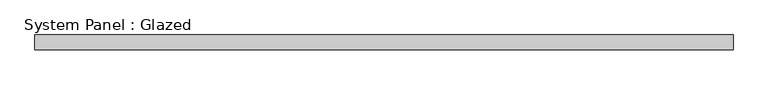
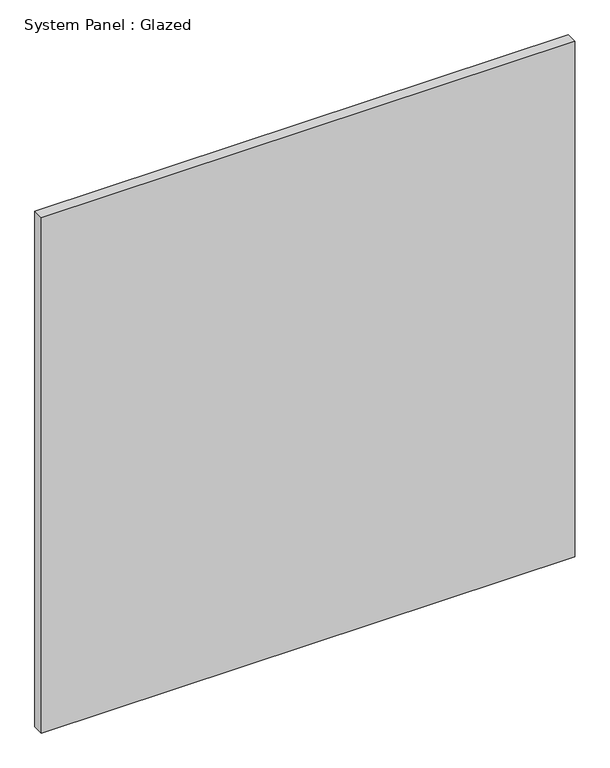
"""IFC4 building model written with IfcOpenShell, lengths in millimetres: plate geometry, System Panel : Glazed."""

from ifc_helpers import new_model, si_unit, origin, origin_with_axes, place, context, project, spatial, polyline, outline, extrude, source, transform, mapped, element, save


def system_panel_glazed_f6fb2dd6(model_context):
    return source(origin(), model_context, "Body", "SweptSolid", [
        extrude(outline(polyline([(596.9, 19.05), (-596.9, 19.05), (-596.9, 44.45), (596.9, 44.45), (596.9, 19.05)])), origin_with_axes(), (0.0, 0.0, 1.0), 1219.2),
    ])


if __name__ == "__main__":
    model = new_model("IFC4")
    model_context = context("Model", 3, world=origin())
    ifc_project = project(units=[si_unit("LENGTHUNIT", "METRE", prefix="MILLI")], contexts=[model_context])
    site = spatial("IfcSite", under=ifc_project)
    building = spatial("IfcBuilding", under=site)
    placement = place(None, origin())
    system_panel_glazed_shape = system_panel_glazed_f6fb2dd6(model_context)
    element("IfcPlate", 1, ObjectType="System Panel : Glazed", at=placement, inside=building, context=model_context, shape_type="MappedRepresentation", body=[
        mapped(system_panel_glazed_shape, transform((0.0, 0.0, 0.0), x_axis=(1.0, 0.0, 0.0), y_axis=(0.0, 1.0, 0.0), z_axis=(0.0, 0.0, 1.0))),
    ])
    save(model, "model.ifc")

# Revit data of these elements
# Type "System Panel : Glazed"
#   Construction Type Id = "GSP4R"
#   Analytic Construction = "1/8 in Pilkington single glazing"
#   Visual Light Transmittance = 0.9
#   Solar Heat Gain Coefficient = 0.86
#   Heat Transfer Coefficient (U) = 1.18115 BTU/(h·ft²·°F)
# Element 1 (IfcPlate, "System Panel : Glazed")
#   Materials on its faces: "Glass"
# Materials
#   "Glass": class "Glass", colour RGB 0 128 192, transparency 0.75, Description = "Soda Lime Glass", Cost = 0
